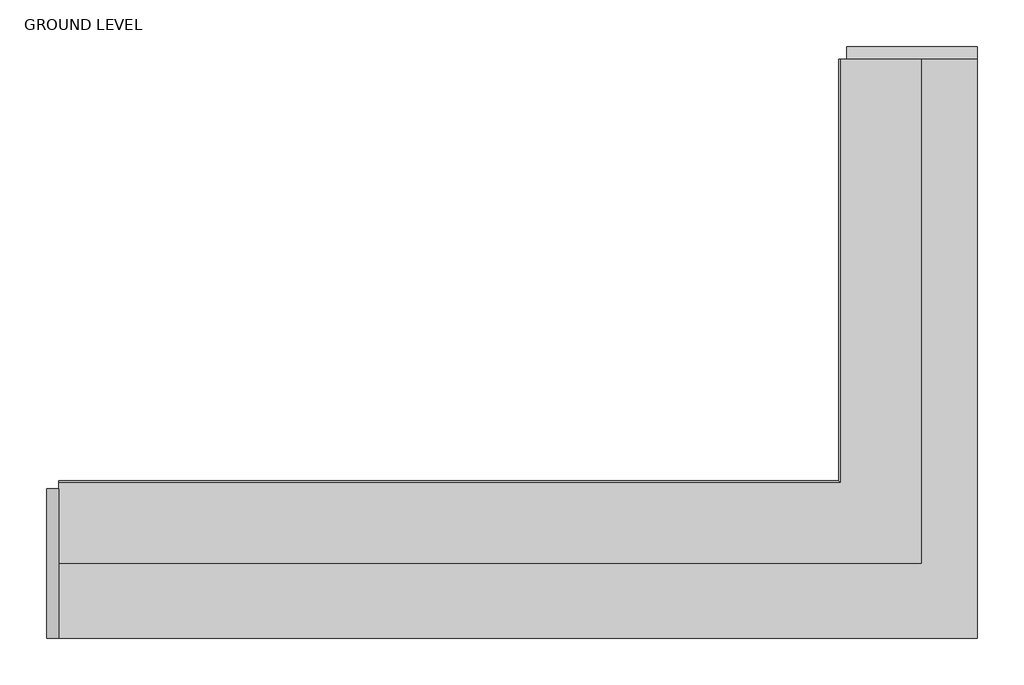
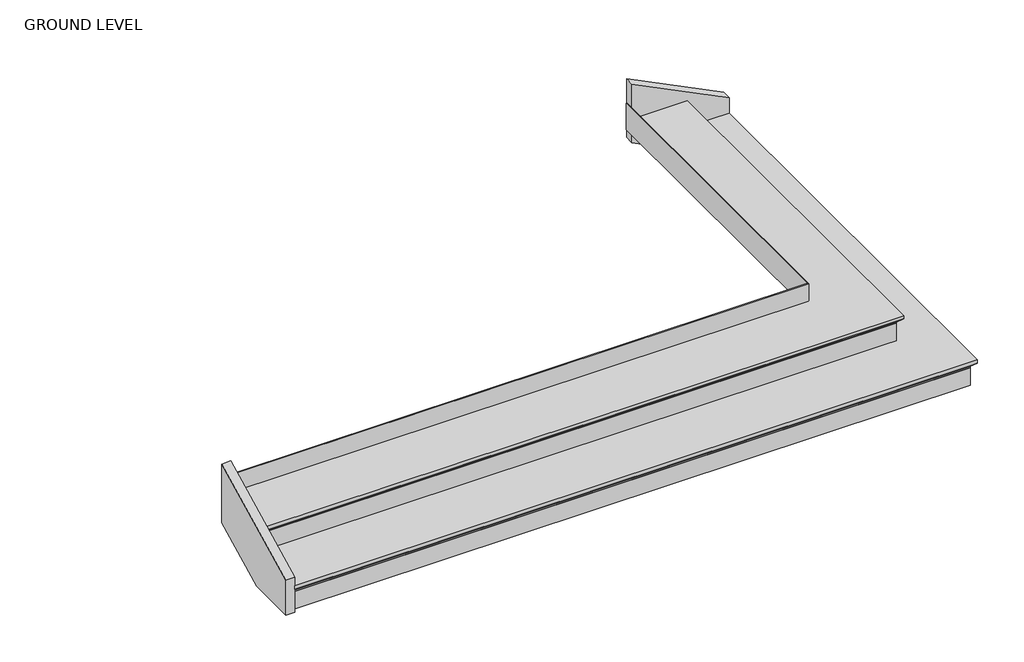
# One storey: 2 members, 1 stair flight.
"""IFC4 building model written with IfcOpenShell, lengths in millimetres."""

from ifc_helpers import new_model, si_unit, frame, origin, place, context, project, spatial, polyline, outline, extrude, transform, mapped, element, save
from components import stair_flight_046a4295

model = new_model("IFC4")

# Units and contexts
model_context = context("Model", 3, world=origin())
ifc_project = project(units=[si_unit("LENGTHUNIT", "METRE", prefix="MILLI")], contexts=[model_context])

# Site, building, storey
site = spatial("IfcSite", under=ifc_project)
building = spatial("IfcBuilding", under=site)
storey = spatial("IfcBuildingStorey", under=building, Name="GROUND LEVEL", Elevation=0.0)

# Members
placement = place(None, origin())
element("IfcMember", 1, ObjectType="Stringer - 2\" Width", at=placement, inside=storey, context=model_context, shape_type="SweptSolid", body=[
    extrude(outline(polyline([(-8599.2948807, 0.0), (-8599.2948807, 203.1066015), (-7989.6948807, 507.9066015), (-7989.6948807, 167.1298417), (-8323.9545641, 0.0), (-8599.2948807, 0.0)])), frame((-5066.0206632, 0.0, 0.0), z_axis=(1.0, 0.0, 0.0), x_axis=(0.0, 1.0, 0.0)), (0.0, 0.0, 1.0), 50.8),
])
element("IfcMember", 2, ObjectType="Stringer - 2\" Width", at=placement, inside=storey, context=model_context, shape_type="SweptSolid", body=[
    extrude(outline(polyline([(0.0, -1268.7206632), (241.2066015, -1268.7206632), (507.9066015, -1802.1206632), (167.1298417, -1802.1206632), (0.0, -1467.8609797), (0.0, -1268.7206632)])), frame((0.0, -6237.0948807, 0.0), z_axis=(0.0, 1.0, 0.0), x_axis=(0.0, 0.0, 1.0)), (0.0, 0.0, 1.0), 50.8),
])

# Stair flight
stair_flight_shape = stair_flight_046a4295(model_context)
element("IfcStairFlight", 3, ObjectType="2\" Tread 1\" Nosing 1/4\" Riser", at=placement, inside=storey, context=model_context, shape_type="MappedRepresentation", body=[
    mapped(stair_flight_shape, transform((0.0, 0.0, 0.0), x_axis=(1.0, 0.0, 0.0), y_axis=(0.0, 1.0, 0.0), z_axis=(0.0, 0.0, 1.0))),
])

save(model, "model.ifc")

# Revit data of these elements
# Elements 1, 2 (IfcMember, "Stringer - 2\" Width")
#   Phase Created = New Construction
# Element 3 (IfcStairFlight, "2\" Tread 1\" Nosing 1/4\" Riser")
#   Phase Created = New Construction
